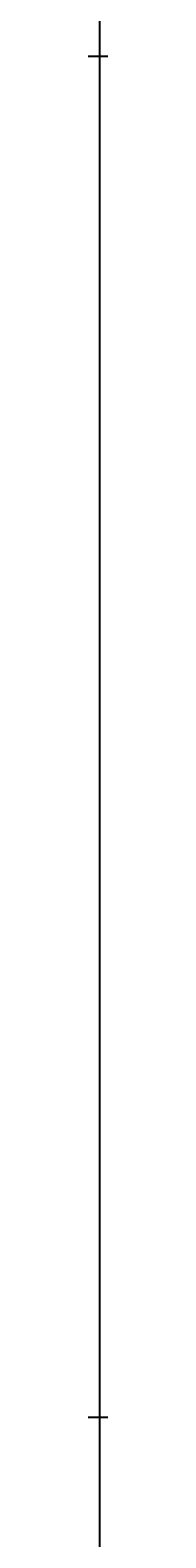
# Model space of a CAD drawing. Units: inches. Extents: x 35362 to 73946, y 43607 to 67532.
# Tile 24 of 134: x 48373 to 48373, y 46091 to 46564. Entities that reach past the tile are written whole.
import ezdxf

# ---------------------------------------------------------------- set-up
doc = ezdxf.new("R2010")
doc.units = ezdxf.units.IN
doc.header["$MEASUREMENT"] = 0
doc.layers.add('A-ANNO-DIMS', color=2, linetype='Continuous', lineweight=18)
doc.styles.get("Standard").update_dxf_attribs({"font": 'arial.ttf'})
doc.dimstyles.get("Standard").update_dxf_attribs({"dimtxt": 0.18, "dimasz": 0.18, "dimexe": 0.18, "dimexo": 0.0625, "dimgap": 0.09, "dimtad": 0, "dimtih": 1, "dimtoh": 1, "dimdec": 4, "dimzin": 0, "dimdsep": 46, "dimtxsty": 'Standard', "dimcen": 0.09, "dimadec": 0, "dimazin": 0, "dimtfac": 1, "dimtdec": 4, "dimtofl": 0, "dimtmove": 0, "dimatfit": 3, "dimfxl": 1, "dimtolj": 1, "dimtzin": 0, "dimarcsym": 0})

# ---------------------------------------------------------------- blocks, each defined once
blk = doc.blocks.new('*D5')
at = {"layer": 'A-ANNO-DIMS', "color": 0, "lineweight": -2, "transparency": 16777216}
for p, q in [((37121.95, 46919.32), (37121.95, 43606.68)), ((69871.5, 45449.83), (69871.5, 43606.68)), ((37122.13, 43606.86), (53496.29, 43606.86)), ((69871.32, 43606.86), (53497.15, 43606.86))]:
    blk.add_line(p, q, dxfattribs=at)
at = {"layer": 'A-ANNO-DIMS', "color": 0, "transparency": 16777216}
for points in [[(37122.13, 43606.89), (37122.13, 43606.83), (37121.95, 43606.86)], [(69871.32, 43606.89), (69871.32, 43606.83), (69871.5, 43606.86)]]:
    blk.add_solid(points, dxfattribs=at)
at = {"layer": 'Defpoints', "color": 0, "transparency": 16777216}
for p in [(37121.95, 46919.38), (69871.5, 45449.89), (69871.5, 43606.86)]:
    blk.add_point(p, dxfattribs=at)
at = {"layer": 'A-ANNO-DIMS', "color": 0, "transparency": 16777216, "insert": (53496.72, 43606.86), "char_height": 0.18, "attachment_point": 5}
blk.add_mtext('\\A1;32750', dxfattribs=at)
blk = doc.blocks.new('*D11')
at = {"layer": 'A-ANNO-DIMS', "color": 0, "lineweight": -2, "transparency": 16777216}
for p, q in [((47978.66, 56028.77), (47978.66, 43606.68)), ((53109.76, 56028.77), (53109.76, 43606.68)), ((47978.84, 43606.86), (50543.87, 43606.86)), ((53109.58, 43606.86), (50544.55, 43606.86))]:
    blk.add_line(p, q, dxfattribs=at)
at = {"layer": 'A-ANNO-DIMS', "color": 0, "transparency": 16777216}
for points in [[(47978.84, 43606.89), (47978.84, 43606.83), (47978.66, 43606.86)], [(53109.58, 43606.89), (53109.58, 43606.83), (53109.76, 43606.86)]]:
    blk.add_solid(points, dxfattribs=at)
at = {"layer": 'Defpoints', "color": 0, "transparency": 16777216}
for p in [(47978.66, 56028.84), (53109.76, 56028.84), (53109.76, 43606.86)]:
    blk.add_point(p, dxfattribs=at)
at = {"layer": 'A-ANNO-DIMS', "color": 0, "transparency": 16777216, "insert": (50544.21, 43606.86), "char_height": 0.18, "attachment_point": 5}
blk.add_mtext('\\A1;5131', dxfattribs=at)
blk = doc.blocks.new('*D27')
at = {"layer": 'A-ANNO-DIMS', "color": 0, "lineweight": -2, "transparency": 16777216}
for p, q in [((47978.66, 56028.77), (47978.66, 43606.68)), ((48373.49, 53428.96), (48373.49, 43606.68)), ((47978.84, 43606.86), (48175.68, 43606.86)), ((48373.31, 43606.86), (48176.47, 43606.86))]:
    blk.add_line(p, q, dxfattribs=at)
at = {"layer": 'A-ANNO-DIMS', "color": 0, "transparency": 16777216}
for points in [[(47978.84, 43606.89), (47978.84, 43606.83), (47978.66, 43606.86)], [(48373.31, 43606.89), (48373.31, 43606.83), (48373.49, 43606.86)]]:
    blk.add_solid(points, dxfattribs=at)
at = {"layer": 'Defpoints', "color": 0, "transparency": 16777216}
for p in [(47978.66, 56028.84), (48373.49, 53429.02), (48373.49, 43606.86)]:
    blk.add_point(p, dxfattribs=at)
at = {"layer": 'A-ANNO-DIMS', "color": 0, "transparency": 16777216, "insert": (48176.08, 43606.86), "char_height": 0.18, "attachment_point": 5}
blk.add_mtext('\\A1;394.8', dxfattribs=at)
blk = doc.blocks.new('*D67')
at = {"layer": 'A-ANNO-DIMS', "color": 0, "lineweight": -2, "transparency": 16777216}
for p, q in [((56873.54, 53351.53), (35361.77, 53351.53)), ((35361.95, 53351.35), (35361.95, 49400.89)), ((35361.95, 45450.07), (35361.95, 49400.53)), ((53793.58, 45449.89), (35361.77, 45449.89))]:
    blk.add_line(p, q, dxfattribs=at)
at = {"layer": 'A-ANNO-DIMS', "color": 0, "transparency": 16777216}
for points in [[(35361.92, 53351.35), (35361.98, 53351.35), (35361.95, 53351.53)], [(35361.92, 45450.07), (35361.98, 45450.07), (35361.95, 45449.89)]]:
    blk.add_solid(points, dxfattribs=at)
at = {"layer": 'Defpoints', "color": 0, "transparency": 16777216}
for p in [(35361.95, 53351.53), (56873.6, 53351.53), (53793.64, 45449.89)]:
    blk.add_point(p, dxfattribs=at)
at = {"layer": 'A-ANNO-DIMS', "color": 0, "transparency": 16777216, "insert": (35361.95, 49400.71), "char_height": 0.18, "attachment_point": 5}
blk.add_mtext('\\A1;7901.6', dxfattribs=at)
blk = doc.blocks.new('*D76')
at = {"layer": 'A-ANNO-DIMS', "color": 0, "lineweight": -2, "transparency": 16777216}
for p, q in [((54052.84, 46555.29), (35361.77, 46555.29)), ((35361.95, 46555.11), (35361.95, 46342.27)), ((35361.95, 46129.06), (35361.95, 46341.9)), ((53793.58, 46128.88), (35361.77, 46128.88))]:
    blk.add_line(p, q, dxfattribs=at)
at = {"layer": 'A-ANNO-DIMS', "color": 0, "transparency": 16777216}
for points in [[(35361.92, 46555.11), (35361.98, 46555.11), (35361.95, 46555.29)], [(35361.92, 46129.06), (35361.98, 46129.06), (35361.95, 46128.88)]]:
    blk.add_solid(points, dxfattribs=at)
at = {"layer": 'Defpoints', "color": 0, "transparency": 16777216}
for p in [(35361.95, 46555.29), (54052.9, 46555.29), (53793.64, 46128.88)]:
    blk.add_point(p, dxfattribs=at)
at = {"layer": 'A-ANNO-DIMS', "color": 0, "transparency": 16777216, "insert": (35361.95, 46342.09), "char_height": 0.18, "attachment_point": 5}
blk.add_mtext('\\A1;426.4', dxfattribs=at)
blk = doc.blocks.new('*D90')
at = {"layer": 'A-ANNO-DIMS', "color": 0, "lineweight": -2, "transparency": 16777216}
for p, q in [((53707.72, 47291.29), (35361.77, 47291.29)), ((35361.95, 47291.11), (35361.95, 46710.26)), ((35361.95, 46129.06), (35361.95, 46709.9)), ((53793.58, 46128.88), (35361.77, 46128.88))]:
    blk.add_line(p, q, dxfattribs=at)
at = {"layer": 'A-ANNO-DIMS', "color": 0, "transparency": 16777216}
for points in [[(35361.92, 47291.11), (35361.98, 47291.11), (35361.95, 47291.29)], [(35361.92, 46129.06), (35361.98, 46129.06), (35361.95, 46128.88)]]:
    blk.add_solid(points, dxfattribs=at)
at = {"layer": 'Defpoints', "color": 0, "transparency": 16777216}
for p in [(53707.78, 47291.29), (35361.95, 46128.88), (53793.64, 46128.88)]:
    blk.add_point(p, dxfattribs=at)
at = {"layer": 'A-ANNO-DIMS', "color": 0, "transparency": 16777216, "insert": (35361.95, 46710.08), "char_height": 0.18, "attachment_point": 5}
blk.add_mtext('\\A1;1162.4', dxfattribs=at)

msp = doc.modelspace()

# ---------------------------------------------------------------- dimensions: what is measured, and where the dimension line sits
at = {"layer": 'A-ANNO-DIMS'}
for base, p1, p2, override, picture, middle in [((53109.76, 43606.859), (47978.665, 56028.836), (53109.76, 56028.836), {"dimdec": 0, "dimlfac": 1, "dimrnd": 0, "dimzin": 0, "dimdsep": 46, "dimlunit": 2}, '*D11', (50544.212, 43606.859)), ((48373.492, 43606.859), (47978.665, 56028.836), (48373.492, 53429.019), {"dimdec": 1, "dimlfac": 1, "dimrnd": 0, "dimzin": 0, "dimdsep": 46, "dimlunit": 2}, '*D27', (48176.078, 43606.859)), ((69871.496, 43606.859), (37121.949, 46919.381), (69871.496, 45449.894), {"dimdec": 0, "dimlfac": 1, "dimrnd": 0, "dimzin": 0, "dimdsep": 46, "dimlunit": 2}, '*D5', (53496.723, 43606.859))]:
    dim = msp.add_linear_dim(base=base, p1=p1, p2=p2, dimstyle='Standard', override=override, dxfattribs=at)
    dim.commit()
    dim.dimension.update_dxf_attribs({"geometry": picture, "text_midpoint": middle})
for base, p1, p2, picture, middle in [((35361.949, 53351.529), (53793.638, 45449.894), (56873.602, 53351.529), '*D67', (35361.949, 49400.712)), ((35361.949, 46128.878), (53707.781, 47291.285), (53793.638, 46128.878), '*D90', (35361.949, 46710.081)), ((35361.949, 46555.293), (53793.638, 46128.878), (54052.899, 46555.293), '*D76', (35361.949, 46342.086))]:
    dim = msp.add_linear_dim(base=base, p1=p1, p2=p2, angle=90, dimstyle='Standard', override={"dimdec": 1, "dimlfac": 1, "dimrnd": 0, "dimzin": 0, "dimdsep": 46, "dimlunit": 2}, dxfattribs=at)
    dim.commit()
    dim.dimension.update_dxf_attribs({"geometry": picture, "text_midpoint": middle})

doc.saveas('drawing.dxf')
